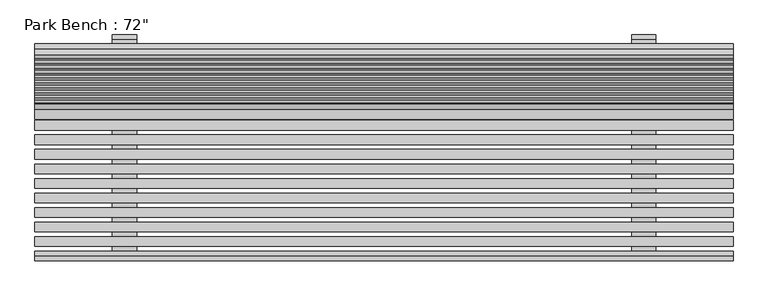
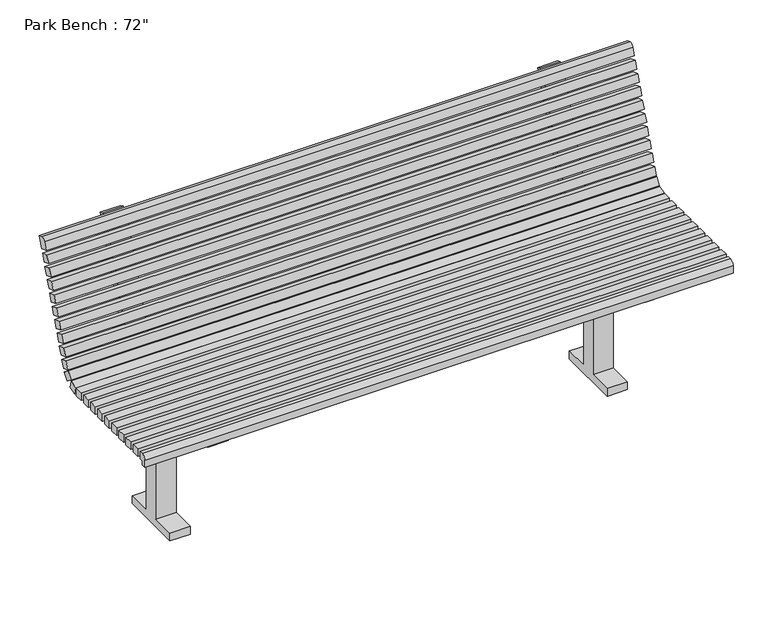
"""IFC4 building model written with IfcOpenShell, lengths in millimetres: geographic element geometry."""

from ifc_helpers import new_model, si_unit, point, frame, frame_2d, origin, place, context, project, spatial, polyline, circle_curve, trimmed, segment, composite_curve, outline, extrude, source, transform, mapped, element, save


def geographic_element_235d1464(model_context):
    return source(origin(), model_context, "Body", "SweptSolid", [
        extrude(outline(polyline([(914.4, -255.4337104), (914.4, -280.8337104), (-914.4, -280.8337104), (-914.4, -255.4337104), (914.4, -255.4337104)])), frame((0.0, 0.0, 457.2), z_axis=(0.0, 0.0, 1.0), x_axis=(1.0, 0.0, 0.0)), (0.0, 0.0, 1.0), 25.4),
        extrude(outline(polyline([(914.4, -217.3337104), (914.4, -242.7337104), (-914.4, -242.7337104), (-914.4, -217.3337104), (914.4, -217.3337104)])), frame((0.0, 0.0, 457.2), z_axis=(0.0, 0.0, 1.0), x_axis=(1.0, 0.0, 0.0)), (0.0, 0.0, 1.0), 25.4),
        extrude(outline(polyline([(914.4, -179.2337104), (914.4, -204.6337104), (-914.4, -204.6337104), (-914.4, -179.2337104), (914.4, -179.2337104)])), frame((0.0, 0.0, 457.2), z_axis=(0.0, 0.0, 1.0), x_axis=(1.0, 0.0, 0.0)), (0.0, 0.0, 1.0), 25.4),
        extrude(outline(polyline([(914.4, -141.1337104), (914.4, -166.5337104), (-914.4, -166.5337104), (-914.4, -141.1337104), (914.4, -141.1337104)])), frame((0.0, 0.0, 457.2), z_axis=(0.0, 0.0, 1.0), x_axis=(1.0, 0.0, 0.0)), (0.0, 0.0, 1.0), 25.4),
        extrude(outline(polyline([(914.4, -103.0337104), (914.4, -128.4337104), (-914.4, -128.4337104), (-914.4, -103.0337104), (914.4, -103.0337104)])), frame((0.0, 0.0, 457.2), z_axis=(0.0, 0.0, 1.0), x_axis=(1.0, 0.0, 0.0)), (0.0, 0.0, 1.0), 25.4),
        extrude(outline(polyline([(914.4, -64.9337104), (914.4, -90.3337104), (-914.4, -90.3337104), (-914.4, -64.9337104), (914.4, -64.9337104)])), frame((0.0, 0.0, 457.2), z_axis=(0.0, 0.0, 1.0), x_axis=(1.0, 0.0, 0.0)), (0.0, 0.0, 1.0), 25.4),
        extrude(outline(polyline([(914.4, -26.8337104), (914.4, -52.2337104), (-914.4, -52.2337104), (-914.4, -26.8337104), (914.4, -26.8337104)])), frame((0.0, 0.0, 457.2), z_axis=(0.0, 0.0, 1.0), x_axis=(1.0, 0.0, 0.0)), (0.0, 0.0, 1.0), 25.4),
        extrude(outline(polyline([(914.4, 11.2662896), (914.4, -14.1337104), (-914.4, -14.1337104), (-914.4, 11.2662896), (914.4, 11.2662896)])), frame((0.0, 0.0, 457.2), z_axis=(0.0, 0.0, 1.0), x_axis=(1.0, 0.0, 0.0)), (0.0, 0.0, 1.0), 25.4),
        extrude(outline(polyline([(914.4, 49.3662896), (914.4, 23.9662896), (-914.4, 23.9662896), (-914.4, 49.3662896), (914.4, 49.3662896)])), frame((0.0, 0.0, 457.2), z_axis=(0.0, 0.0, 1.0), x_axis=(1.0, 0.0, 0.0)), (0.0, 0.0, 1.0), 25.4),
        extrude(outline(composite_curve([segment(polyline([(-304.8, 457.2), (-304.8, 444.5), (-318.9337104, 444.5), (-318.9337104, 468.3125)]), True, "CONTINUOUS"), segment(trimmed(circle_curve(frame_2d((-304.6462104, 468.3125)), 14.2875), [point((-318.9337104, 468.3125))], [point((-304.6462104, 482.6))], False, "CARTESIAN"), True, "CONTINUOUS"), segment(polyline([(-304.6462104, 482.6), (-293.5337104, 482.6), (-293.5337104, 457.2), (-304.8, 457.2)]), True, "CONTINUOUS")], self_intersect=False)), frame((-914.4, 0.0, 0.0), z_axis=(1.0, 0.0, 0.0), x_axis=(0.0, 1.0, 0.0)), (0.0, 0.0, 1.0), 1828.8),
        extrude(outline(polyline([(0.0, -25.4), (0.0, 0.0), (1828.8, 0.0), (1828.8, -25.4), (0.0, -25.4)])), frame((914.4, 121.2738625, 585.5181247), z_axis=(0.0, 0.342020143325687, 0.9396926207859018), x_axis=(-1.0, 0.0, 0.0)), (0.0, 0.0, 1.0), 25.4),
        extrude(outline(polyline([(0.0, -25.4), (0.0, 0.0), (1828.8, 0.0), (1828.8, -25.4), (0.0, -25.4)])), frame((914.4, 134.30483, 621.3204136), z_axis=(0.0, 0.34202014332568254, 0.9396926207859034), x_axis=(-1.0, 0.0, 0.0)), (0.0, 0.0, 1.0), 25.4),
        extrude(outline(polyline([(0.0, -25.3999999), (0.0, 0.0), (1828.8, 0.0), (1828.8, -25.3999999), (0.0, -25.3999999)])), frame((914.4, 95.2119276, 513.913547), z_axis=(0.0, 0.34202014332568254, 0.9396926207859034), x_axis=(-1.0, 0.0, 0.0)), (0.0, 0.0, 1.0), 25.4),
        extrude(outline(polyline([(0.0, -25.4000001), (0.0, 0.0), (1828.8, 0.0), (1828.8, -25.4000001), (0.0, -25.4000001)])), frame((914.4, 108.242895, 549.7158359), z_axis=(0.0, 0.34202014332567804, 0.9396926207859051), x_axis=(-1.0, 0.0, 0.0)), (0.0, 0.0, 1.0), 25.4),
        extrude(outline(polyline([(0.0, -25.4), (0.0, 0.0), (1828.8, 0.0), (1828.8, -25.4), (0.0, -25.4)])), frame((914.4, 173.3977323, 728.7272801), z_axis=(0.0, 0.34202014332568337, 0.9396926207859031), x_axis=(-1.0, 0.0, 0.0)), (0.0, 0.0, 1.0), 25.4),
        extrude(outline(polyline([(0.0, -25.4000001), (0.0, 0.0), (1828.8, 0.0), (1828.8, -25.4000001), (0.0, -25.4000001)])), frame((914.4, 186.4286998, 764.529569), z_axis=(0.0, 0.3420201433256829, 0.9396926207859032), x_axis=(-1.0, 0.0, 0.0)), (0.0, 0.0, 1.0), 25.4),
        extrude(outline(polyline([(0.0, -25.4), (0.0, 0.0), (1828.8, 0.0), (1828.8, -25.4), (0.0, -25.4)])), frame((914.4, 147.3357974, 657.1227024), z_axis=(0.0, 0.3420201433256776, 0.9396926207859052), x_axis=(-1.0, 0.0, 0.0)), (0.0, 0.0, 1.0), 25.4),
        extrude(outline(polyline([(0.0, -25.4), (0.0, 0.0), (1828.8, 0.0), (1828.8, -25.4), (0.0, -25.4)])), frame((914.4, 160.3667649, 692.9249913), z_axis=(0.0, 0.34202014332568254, 0.9396926207859034), x_axis=(-1.0, 0.0, 0.0)), (0.0, 0.0, 1.0), 25.4),
        extrude(outline(polyline([(0.0, -25.3999999), (0.0, 0.0), (1828.8, 0.0), (1828.8, -25.3999999), (0.0, -25.3999999)])), frame((914.4, 199.4596673, 800.3318578), z_axis=(0.0, 0.3420201433256774, 0.9396926207859052), x_axis=(-1.0, 0.0, 0.0)), (0.0, 0.0, 1.0), 25.4),
        extrude(outline(composite_curve([segment(polyline([(249.3897948, 863.2491239), (236.3588273, 827.4468351), (212.4906347, 836.1341467), (221.1779464, 860.0023393)]), True, "CONTINUOUS"), segment(trimmed(circle_curve(frame_2d((233.1120426, 855.6586834)), 12.7), [point((221.1779464, 860.0023393))], [point((237.4556985, 867.5927797))], False, "CARTESIAN"), True, "CONTINUOUS"), segment(polyline([(237.4556985, 867.5927797), (249.3897948, 863.2491239)]), True, "CONTINUOUS")], self_intersect=False)), frame((-914.4, 0.0, 0.0), z_axis=(1.0, 0.0, 0.0), x_axis=(0.0, 1.0, 0.0)), (0.0, 0.0, 1.0), 1828.8),
        extrude(outline(polyline([(0.0, -25.4), (0.0, 0.0), (1828.8, 0.0), (1828.8, -25.4), (0.0, -25.4)])), frame((914.4, 78.7855779, 490.7267336), z_axis=(0.0, 0.5735764363510742, 0.8191520442889721), x_axis=(-1.0, 0.0, 0.0)), (0.0, 0.0, 1.0), 25.4),
        extrude(outline(polyline([(0.0, -25.4), (0.0, 0.0), (1828.8, 0.0), (1828.8, -25.4), (0.0, -25.4)])), frame((914.4, 59.0817015, 457.2297909), z_axis=(0.0, -0.2588190451024684, 0.9659258262890824), x_axis=(-1.0, 0.0, 0.0)), (0.0, 0.0, 1.0), 25.4),
        extrude(outline(composite_curve([segment(polyline([(-101.6, 25.4), (-25.4, 25.4), (-25.4, 431.8), (-304.8, 431.8), (-304.8, 457.2), (57.1368213, 457.2)]), True, "CONTINUOUS"), segment(trimmed(circle_curve(frame_2d((57.1368213, 520.7)), 63.5), [point((57.1368213, 457.2))], [point((116.8073027, 498.9817209))], True, "CARTESIAN"), True, "CONTINUOUS"), segment(polyline([(116.8073027, 498.9817209), (244.9406421, 851.0251774)]), True, "CONTINUOUS"), segment(trimmed(circle_curve(frame_2d((256.8747384, 846.6815216)), 12.7), [point((244.9406421, 851.0251774))], [point((261.2183942, 858.6156178))], False, "CARTESIAN"), True, "CONTINUOUS"), segment(polyline([(261.2183942, 858.6156178), (273.1524905, 854.271962), (140.6754953, 490.2944093)]), True, "CONTINUOUS"), segment(trimmed(circle_curve(frame_2d((57.1368213, 520.7)), 88.9), [point((140.6754953, 490.2944093))], [point((57.1368213, 431.8))], False, "CARTESIAN"), True, "CONTINUOUS"), segment(polyline([(57.1368213, 431.8), (25.4, 431.8), (25.4, 25.4), (101.6, 25.4), (101.6, 0.0), (-101.6, 0.0), (-101.6, 25.4)]), True, "CONTINUOUS")], self_intersect=False)), frame((648.3736591, 0.0, 0.0), z_axis=(1.0, 0.0, 0.0), x_axis=(0.0, 1.0, 0.0)), (0.0, 0.0, 1.0), 62.8263409),
        extrude(outline(composite_curve([segment(polyline([(-101.6, 25.4), (-25.4, 25.4), (-25.4, 431.8), (-304.8, 431.8), (-304.8, 457.2), (57.1368213, 457.2)]), True, "CONTINUOUS"), segment(trimmed(circle_curve(frame_2d((57.1368213, 520.7)), 63.5), [point((57.1368213, 457.2))], [point((116.8073027, 498.9817209))], True, "CARTESIAN"), True, "CONTINUOUS"), segment(polyline([(116.8073027, 498.9817209), (244.9406421, 851.0251774)]), True, "CONTINUOUS"), segment(trimmed(circle_curve(frame_2d((256.8747384, 846.6815216)), 12.7), [point((244.9406421, 851.0251774))], [point((261.2183942, 858.6156178))], False, "CARTESIAN"), True, "CONTINUOUS"), segment(polyline([(261.2183942, 858.6156178), (273.1524905, 854.271962), (140.6754953, 490.2944093)]), True, "CONTINUOUS"), segment(trimmed(circle_curve(frame_2d((57.1368213, 520.7)), 88.9), [point((140.6754953, 490.2944093))], [point((57.1368213, 431.8))], False, "CARTESIAN"), True, "CONTINUOUS"), segment(polyline([(57.1368213, 431.8), (25.4, 431.8), (25.4, 25.4), (101.6, 25.4), (101.6, 0.0), (-101.6, 0.0), (-101.6, 25.4)]), True, "CONTINUOUS")], self_intersect=False)), frame((-711.2, 0.0, 0.0), z_axis=(1.0, 0.0, 0.0), x_axis=(0.0, 1.0, 0.0)), (0.0, 0.0, 1.0), 63.8916859),
    ])


if __name__ == "__main__":
    model = new_model("IFC4")
    model_context = context("Model", 3, world=origin())
    ifc_project = project(units=[si_unit("LENGTHUNIT", "METRE", prefix="MILLI")], contexts=[model_context])
    site = spatial("IfcSite", under=ifc_project)
    building = spatial("IfcBuilding", under=site)
    placement = place(None, origin())
    geographic_element_shape = geographic_element_235d1464(model_context)
    element("IfcGeographicElement", 1, ObjectType="Park Bench : 72\"", at=placement, inside=building, context=model_context, shape_type="MappedRepresentation", body=[
        mapped(geographic_element_shape, transform((0.0, 0.0, 0.0), x_axis=(1.0, 0.0, 0.0), y_axis=(0.0, 1.0, 0.0), z_axis=(0.0, 0.0, 1.0))),
    ])
    save(model, "model.ifc")

# Revit data of these elements
# Type "Park Bench : 72\""
#   Length = 6' - 0"
#   Seat Material = Wood - Teak
#   Frame Material = Steel, Paint Finish, Dark Gray, Matte
# Element 1 (IfcGeographicElement, "Park Bench : 72\"")
#   Materials on its faces: "Wood - Teak", "Steel, Paint Finish, Dark Gray, Matte"
# Materials
#   "Wood - Teak": class "Wood", colour RGB 120 73 19, transparency 0
#   "Steel, Paint Finish, Dark Gray, Matte": class "Metal", colour RGB 98 98 98, transparency 0, Description = "Steel, paint finish, dark gray, matte", Cost = 0
